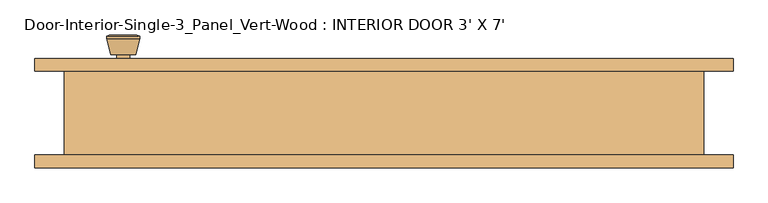
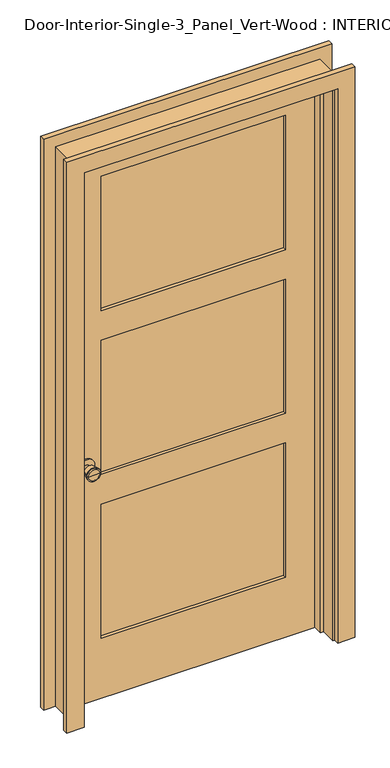
"""IFC4 building model written with IfcOpenShell, lengths in millimetres: door geometry, Door-Interior-Single-3_Panel_Vert-Wood : INTERIOR DOOR 3' X 7'."""

from ifc_helpers import new_model, si_unit, point, frame, frame_2d, origin, place, context, project, spatial, polyline, circle_curve, trimmed, segment, composite_curve, outline, extrude, faceted_brep, source, transform, mapped, element, save
from ifc_brep_helpers import plane_surface, cylinder_surface, revolved_surface, advanced_brep


def door_interior_single_3_panel_vert_wood_interior_door_3_x_7_5540447a(model_context):
    return source(origin(), model_context, "Body", "SolidModel", [
        advanced_brep(
        [(-393.7, 19.4, 914.4), (-383.7, 19.4, 914.4), (-403.7, 19.4, 914.4), (-373.2241324, -29.6, 914.4), (-393.7, -29.6, 914.4), (-414.1758676, -29.6, 914.4), (-368.7, -27.7721319, 914.4), (-418.7, -27.7721319, 914.4), (-368.7, -24.3084537, 914.4), (-418.7, -24.3084537, 914.4), (-375.063764, 0.4, 914.4), (-412.336236, 0.4, 914.4), (-383.7, 0.4, 914.4), (-403.7, 0.4, 914.4)],
        [
            (0, 1),
            (1, 2, circle_curve(frame((-393.7, 19.4, 914.4), z_axis=(0.0, 1.0, 0.0), x_axis=(-1.0, 0.0, 0.0)), 10.0)),
            (2, 0),
            (2, 1, circle_curve(frame((-393.7, 19.4, 914.4), z_axis=(0.0, 1.0, 0.0), x_axis=(-1.0, 0.0, 0.0)), 10.0)),
            (3, 4),
            (4, 5),
            (5, 3, circle_curve(frame((-393.7, -29.6, 914.4), z_axis=(0.0, -1.0, 0.0), x_axis=(-1.0, 0.0, 0.0)), 20.4758676)),
            (3, 5, circle_curve(frame((-393.7, -29.6, 914.4), z_axis=(0.0, -1.0, 0.0), x_axis=(-1.0, 0.0, 0.0)), 20.4758676)),
            (6, 3),
            (5, 7),
            (7, 6, circle_curve(frame((-393.7, -27.7721319, 914.4), z_axis=(0.0, -1.0, 0.0), x_axis=(-1.0, 0.0, 0.0)), 25.0)),
            (6, 7, circle_curve(frame((-393.7, -27.7721319, 914.4), z_axis=(0.0, -1.0, 0.0), x_axis=(-1.0, 0.0, 0.0)), 25.0)),
            (8, 6),
            (7, 9),
            (9, 8, circle_curve(frame((-393.7, -24.3084537, 914.4), z_axis=(0.0, -1.0, 0.0), x_axis=(-1.0, 0.0, 0.0)), 25.0)),
            (8, 9, circle_curve(frame((-393.7, -24.3084537, 914.4), z_axis=(0.0, -1.0, 0.0), x_axis=(-1.0, 0.0, 0.0)), 25.0)),
            (10, 8),
            (9, 11),
            (11, 10, circle_curve(frame((-393.7, 0.4, 914.4), z_axis=(0.0, -1.0, 0.0), x_axis=(-1.0, 0.0, 0.0)), 18.636236)),
            (10, 11, circle_curve(frame((-393.7, 0.4, 914.4), z_axis=(0.0, -1.0, 0.0), x_axis=(-1.0, 0.0, 0.0)), 18.636236)),
            (12, 10),
            (11, 13),
            (13, 12, circle_curve(frame((-393.7, 0.4, 914.4), z_axis=(0.0, -1.0, 0.0), x_axis=(-1.0, 0.0, 0.0)), 10.0)),
            (12, 13, circle_curve(frame((-393.7, 0.4, 914.4), z_axis=(0.0, -1.0, 0.0), x_axis=(-1.0, 0.0, 0.0)), 10.0)),
            (1, 12),
            (13, 2),
        ],
        [
            plane_surface(frame((-393.7, 19.4, 914.4), z_axis=(0.0, 1.0, 0.0), x_axis=(-1.0, 0.0, 0.0))),
            plane_surface(frame((-393.7, -29.6, 914.4), z_axis=(0.0, -1.0, 0.0), x_axis=(-1.0, 0.0, 0.0))),
            revolved_surface(polyline([(-414.1758676, -29.6, 914.4), (-418.7, -27.7721319, 914.4)]), (-393.7, 19.4, 914.4), (0.0, 1.0, 0.0)),
            cylinder_surface(frame((-393.7, 19.4, 914.4), z_axis=(0.0, 1.0, 0.0), x_axis=(-1.0, 0.0, 0.0)), 25.0),
            revolved_surface(polyline([(-418.7, -24.3084537, 914.4), (-412.336236, 0.4, 914.4)]), (-393.7, 19.4, 914.4), (0.0, 1.0, 0.0)),
            plane_surface(frame((-393.7, 0.4, 914.4), z_axis=(0.0, 1.0, 0.0), x_axis=(-1.0, 0.0, 0.0))),
            cylinder_surface(frame((-393.7, 19.4, 914.4), z_axis=(0.0, 1.0, 0.0), x_axis=(-1.0, 0.0, 0.0)), 10.0),
        ],
        [
            (0, [[1, 2, 3]]),
            (0, [[-3, 4, -1]]),
            (1, [[5, 6, 7]]),
            (1, [[-6, -5, 8]]),
            (2, [[9, -7, 10, 11]]),
            (2, [[-10, -8, -9, 12]]),
            (3, [[13, -11, 14, 15]]),
            (3, [[-14, -12, -13, 16]]),
            (4, [[17, -15, 18, 19]]),
            (4, [[-18, -16, -17, 20]]),
            (5, [[21, -19, 22, 23]]),
            (5, [[-22, -20, -21, 24]]),
            (6, [[25, -23, 26, -2]]),
            (6, [[-26, -24, -25, -4]]),
        ],
    ),
        extrude(outline(composite_curve([segment(trimmed(circle_curve(frame_2d((914.4, -393.7)), 30.0), [point((914.4, -423.7))], [point((914.4, -363.7))], False, "CARTESIAN"), True, "CONTINUOUS"), segment(trimmed(circle_curve(frame_2d((914.4, -393.7)), 30.0), [point((914.4, -363.7))], [point((914.4, -423.7))], False, "CARTESIAN"), True, "CONTINUOUS")], self_intersect=False)), frame((0.0, 19.4, 0.0), z_axis=(0.0, 1.0, 0.0), x_axis=(0.0, 0.0, 1.0)), (0.0, 0.0, 1.0), 6.0),
        advanced_brep(
        [(-393.7, 66.325, 914.4), (-403.7, 66.325, 914.4), (-383.7, 66.325, 914.4), (-373.2241324, 115.325, 914.4), (-414.1758676, 115.325, 914.4), (-393.7, 115.325, 914.4), (-368.7, 113.4971319, 914.4), (-418.7, 113.4971319, 914.4), (-368.7, 110.0334537, 914.4), (-418.7, 110.0334537, 914.4), (-375.063764, 85.325, 914.4), (-412.336236, 85.325, 914.4), (-383.7, 85.325, 914.4), (-403.7, 85.325, 914.4)],
        [
            (0, 1),
            (1, 2, circle_curve(frame((-393.7, 66.325, 914.4), z_axis=(0.0, -1.0, 0.0), x_axis=(-1.0, 0.0, 0.0)), 10.0)),
            (2, 0),
            (2, 1, circle_curve(frame((-393.7, 66.325, 914.4), z_axis=(0.0, -1.0, 0.0), x_axis=(-1.0, 0.0, 0.0)), 10.0)),
            (3, 4, circle_curve(frame((-393.7, 115.325, 914.4), z_axis=(0.0, 1.0, 0.0), x_axis=(-1.0, 0.0, 0.0)), 20.4758676)),
            (4, 5),
            (5, 3),
            (4, 3, circle_curve(frame((-393.7, 115.325, 914.4), z_axis=(0.0, 1.0, 0.0), x_axis=(-1.0, 0.0, 0.0)), 20.4758676)),
            (6, 7, circle_curve(frame((-393.7, 113.4971319, 914.4), z_axis=(0.0, 1.0, 0.0), x_axis=(-1.0, 0.0, 0.0)), 25.0)),
            (7, 4),
            (3, 6),
            (7, 6, circle_curve(frame((-393.7, 113.4971319, 914.4), z_axis=(0.0, 1.0, 0.0), x_axis=(-1.0, 0.0, 0.0)), 25.0)),
            (8, 9, circle_curve(frame((-393.7, 110.0334537, 914.4), z_axis=(0.0, 1.0, 0.0), x_axis=(-1.0, 0.0, 0.0)), 25.0)),
            (9, 7),
            (6, 8),
            (9, 8, circle_curve(frame((-393.7, 110.0334537, 914.4), z_axis=(0.0, 1.0, 0.0), x_axis=(-1.0, 0.0, 0.0)), 25.0)),
            (10, 11, circle_curve(frame((-393.7, 85.325, 914.4), z_axis=(0.0, 1.0, 0.0), x_axis=(-1.0, 0.0, 0.0)), 18.636236)),
            (11, 9),
            (8, 10),
            (11, 10, circle_curve(frame((-393.7, 85.325, 914.4), z_axis=(0.0, 1.0, 0.0), x_axis=(-1.0, 0.0, 0.0)), 18.636236)),
            (12, 13, circle_curve(frame((-393.7, 85.325, 914.4), z_axis=(0.0, 1.0, 0.0), x_axis=(-1.0, 0.0, 0.0)), 10.0)),
            (13, 11),
            (10, 12),
            (13, 12, circle_curve(frame((-393.7, 85.325, 914.4), z_axis=(0.0, 1.0, 0.0), x_axis=(-1.0, 0.0, 0.0)), 10.0)),
            (1, 13),
            (12, 2),
        ],
        [
            plane_surface(frame((-393.7, 66.325, 914.4), z_axis=(0.0, -1.0, 0.0), x_axis=(-1.0, 0.0, 0.0))),
            plane_surface(frame((-393.7, 115.325, 914.4), z_axis=(0.0, 1.0, 0.0), x_axis=(-1.0, 0.0, 0.0))),
            revolved_surface(polyline([(-414.1758676, 115.325, 914.4), (-418.7, 113.4971319, 914.4)]), (-393.7, 66.325, 914.4), (0.0, -1.0, 0.0)),
            cylinder_surface(frame((-393.7, 66.325, 914.4), z_axis=(0.0, -1.0, 0.0), x_axis=(-1.0, 0.0, 0.0)), 25.0),
            revolved_surface(polyline([(-418.7, 110.0334537, 914.4), (-412.336236, 85.325, 914.4)]), (-393.7, 66.325, 914.4), (0.0, -1.0, 0.0)),
            plane_surface(frame((-393.7, 85.325, 914.4), z_axis=(0.0, -1.0, 0.0), x_axis=(-1.0, 0.0, 0.0))),
            cylinder_surface(frame((-393.7, 66.325, 914.4), z_axis=(0.0, -1.0, 0.0), x_axis=(-1.0, 0.0, 0.0)), 10.0),
        ],
        [
            (0, [[1, 2, 3]]),
            (0, [[-3, 4, -1]]),
            (1, [[5, 6, 7]]),
            (1, [[8, -7, -6]]),
            (2, [[9, 10, -5, 11]]),
            (2, [[12, -11, -8, -10]]),
            (3, [[13, 14, -9, 15]]),
            (3, [[16, -15, -12, -14]]),
            (4, [[17, 18, -13, 19]]),
            (4, [[20, -19, -16, -18]]),
            (5, [[21, 22, -17, 23]]),
            (5, [[24, -23, -20, -22]]),
            (6, [[-2, 25, -21, 26]]),
            (6, [[-4, -26, -24, -25]]),
        ],
    ),
        extrude(outline(composite_curve([segment(trimmed(circle_curve(frame_2d((914.4, -393.7)), 30.0), [point((914.4, -423.7))], [point((914.4, -363.7))], False, "CARTESIAN"), True, "CONTINUOUS"), segment(trimmed(circle_curve(frame_2d((914.4, -393.7)), 30.0), [point((914.4, -363.7))], [point((914.4, -423.7))], False, "CARTESIAN"), True, "CONTINUOUS")], self_intersect=False)), frame((0.0, 60.325, 0.0), z_axis=(0.0, 1.0, 0.0), x_axis=(0.0, 0.0, 1.0)), (0.0, 0.0, 1.0), 6.0),
        faceted_brep([(482.6, 60.325, 0.0), (482.6, -66.675, 0.0), (457.2, -66.675, 0.0), (457.2, -9.525, 0.0), (444.5, -9.525, 0.0), (444.5, 25.4, 0.0), (457.2, 25.4, 0.0), (457.2, 60.325, 0.0), (482.6, 60.325, 2159.0), (482.6, -66.675, 2159.0), (-482.6, -66.675, 2159.0), (-482.6, -66.675, 0.0), (-457.2, -66.675, 0.0), (-457.2, -66.675, 2133.6), (457.2, -66.675, 2133.6), (457.2, -9.525, 2133.6), (-457.2, -9.525, 2133.6), (-457.2, -9.525, 0.0), (-444.5, -9.525, 0.0), (-444.5, -9.525, 2120.9), (444.5, -9.525, 2120.9), (444.5, 25.4, 2120.9), (-444.5, 25.4, 2120.9), (-444.5, 25.4, 0.0), (-457.2, 25.4, 0.0), (-457.2, 25.4, 2133.6), (457.2, 25.4, 2133.6), (457.2, 60.325, 2133.6), (-457.2, 60.325, 2133.6), (-457.2, 60.325, 0.0), (-482.6, 60.325, 0.0), (-482.6, 60.325, 2159.0)], [[[0, 1, 2, 3, 4, 5, 6, 7]], [[1, 0, 8, 9]], [[2, 1, 9, 10, 11, 12, 13, 14]], [[3, 2, 14, 15]], [[4, 3, 15, 16, 17, 18, 19, 20]], [[5, 4, 20, 21]], [[6, 5, 21, 22, 23, 24, 25, 26]], [[7, 6, 26, 27]], [[0, 7, 27, 28, 29, 30, 31, 8]], [[9, 8, 31, 10]], [[15, 14, 13, 16]], [[21, 20, 19, 22]], [[27, 26, 25, 28]], [[30, 29, 24, 23, 18, 17, 12, 11]], [[10, 31, 30, 11]], [[16, 13, 12, 17]], [[22, 19, 18, 23]], [[28, 25, 24, 29]]]),
        extrude(outline(polyline([(2133.6, -457.2), (0.0, -457.2), (0.0, 457.2), (2133.6, 457.2), (2133.6, -457.2)]), holes=[polyline([(2014.5375, -336.55), (2014.5375, 336.55), (1496.4833333, 336.55), (1496.4833333, -336.55), (2014.5375, -336.55)]), polyline([(749.8291667, -336.55), (749.8291667, 336.55), (231.775, 336.55), (231.775, -336.55), (749.8291667, -336.55)]), polyline([(1382.1833333, -336.55), (1382.1833333, 336.55), (864.1291667, 336.55), (864.1291667, -336.55), (1382.1833333, -336.55)])]), frame((0.0, 25.4, 0.0), z_axis=(0.0, 1.0, 0.0), x_axis=(0.0, 0.0, 1.0)), (0.0, 0.0, 1.0), 34.925),
        extrude(outline(polyline([(336.55, 37.0416667), (-336.55, 37.0416667), (-336.55, 48.6833333), (336.55, 48.6833333), (336.55, 37.0416667)])), frame((0.0, 0.0, 1496.4833333), z_axis=(0.0, 0.0, 1.0), x_axis=(1.0, 0.0, 0.0)), (0.0, 0.0, 1.0), 518.0541667),
        extrude(outline(polyline([(336.55, 37.0416667), (-336.55, 37.0416667), (-336.55, 48.6833333), (336.55, 48.6833333), (336.55, 37.0416667)])), frame((0.0, 0.0, 231.775), z_axis=(0.0, 0.0, 1.0), x_axis=(1.0, 0.0, 0.0)), (0.0, 0.0, 1.0), 518.0541667),
        extrude(outline(polyline([(336.55, 37.0416667), (-336.55, 37.0416667), (-336.55, 48.6833333), (336.55, 48.6833333), (336.55, 37.0416667)])), frame((0.0, 0.0, 864.1291667), z_axis=(0.0, 0.0, 1.0), x_axis=(1.0, 0.0, 0.0)), (0.0, 0.0, 1.0), 518.0541667),
        extrude(outline(polyline([(0.0, 463.55), (0.0, 527.05), (2203.45, 527.05), (2203.45, -527.05), (0.0, -527.05), (0.0, -463.55), (2139.95, -463.55), (2139.95, 463.55), (0.0, 463.55)])), frame((0.0, 60.325, 0.0), z_axis=(0.0, 1.0, 0.0), x_axis=(0.0, 0.0, 1.0)), (0.0, 0.0, 1.0), 19.05),
        extrude(outline(polyline([(0.0, 463.55), (0.0, 527.05), (2203.45, 527.05), (2203.45, -527.05), (0.0, -527.05), (0.0, -463.55), (2139.95, -463.55), (2139.95, 463.55), (0.0, 463.55)])), frame((0.0, -85.725, 0.0), z_axis=(0.0, 1.0, 0.0), x_axis=(0.0, 0.0, 1.0)), (0.0, 0.0, 1.0), 19.05),
    ])


if __name__ == "__main__":
    model = new_model("IFC4")
    model_context = context("Model", 3, world=origin())
    ifc_project = project(units=[si_unit("LENGTHUNIT", "METRE", prefix="MILLI")], contexts=[model_context])
    site = spatial("IfcSite", under=ifc_project)
    building = spatial("IfcBuilding", under=site)
    placement = place(None, origin())
    door_interior_single_3_panel_vert_wood_interior_door_3_x_7_shape = door_interior_single_3_panel_vert_wood_interior_door_3_x_7_5540447a(model_context)
    element("IfcDoor", 1, ObjectType="Door-Interior-Single-3_Panel_Vert-Wood : INTERIOR DOOR 3' X 7'", at=placement, inside=building, context=model_context, shape_type="MappedRepresentation", body=[
        mapped(door_interior_single_3_panel_vert_wood_interior_door_3_x_7_shape, transform((0.0, 0.0, 0.0), x_axis=(1.0, 0.0, 0.0), y_axis=(0.0, 1.0, 0.0), z_axis=(0.0, 0.0, 1.0))),
    ])
    save(model, "model.ifc")

# Revit data of these elements
# Type "Door-Interior-Single-3_Panel_Vert-Wood : INTERIOR DOOR 3' X 7'"
#   Type Mark = "10"
#   Assembly Code = "C1020300"
#   Analytic Construction = "Wooden"
#   Top Rail = 0' - 4 11/16"
#   Thickness = 0' - 1 3/8"
#   Thermal Resistance (R) = 2.5876 (h·ft²·°F)/BTU
#   Swing Angle [instance default] = 90.00°
#   Stiles = 0' - 4 3/4"
#   Rough Width = 3' - 2"
#   Rough Height = 7' - 1"
#   Intermediate Rail = 0' - 4 1/2"
#   Height = 7' - 0"
#   Width = 3' - 0"
#   Heat Transfer Coefficient (U) = 0.3865 BTU/(h·ft²·°F)
#   Bottom Rail = 0' - 9 1/8"
#   Trim Material = Cherry
#   Panel Material = Cherry
#   Frame Material = Cherry
#   Door Handle Material = Aluminum
#   Visual Light Transmittance = 0
#   Solar Heat Gain Coefficient = 0
#   Wall Closure = (empty or 0)
#   Function = (empty or 0)
# Element 1 (IfcDoor, "Door-Interior-Single-3_Panel_Vert-Wood : INTERIOR DOOR 3' X 7'")
#   Materials on its faces: "Cherry", "Aluminum"
# Materials
#   "Cherry": class "Wood", colour RGB 226 177 128, transparency 0, Description = "Prunus Serotina", Cost = 0
#   "Aluminum": class "Metal", colour RGB 247 247 247, transparency 0, Description = "Aluminum 6061", Cost = 0
